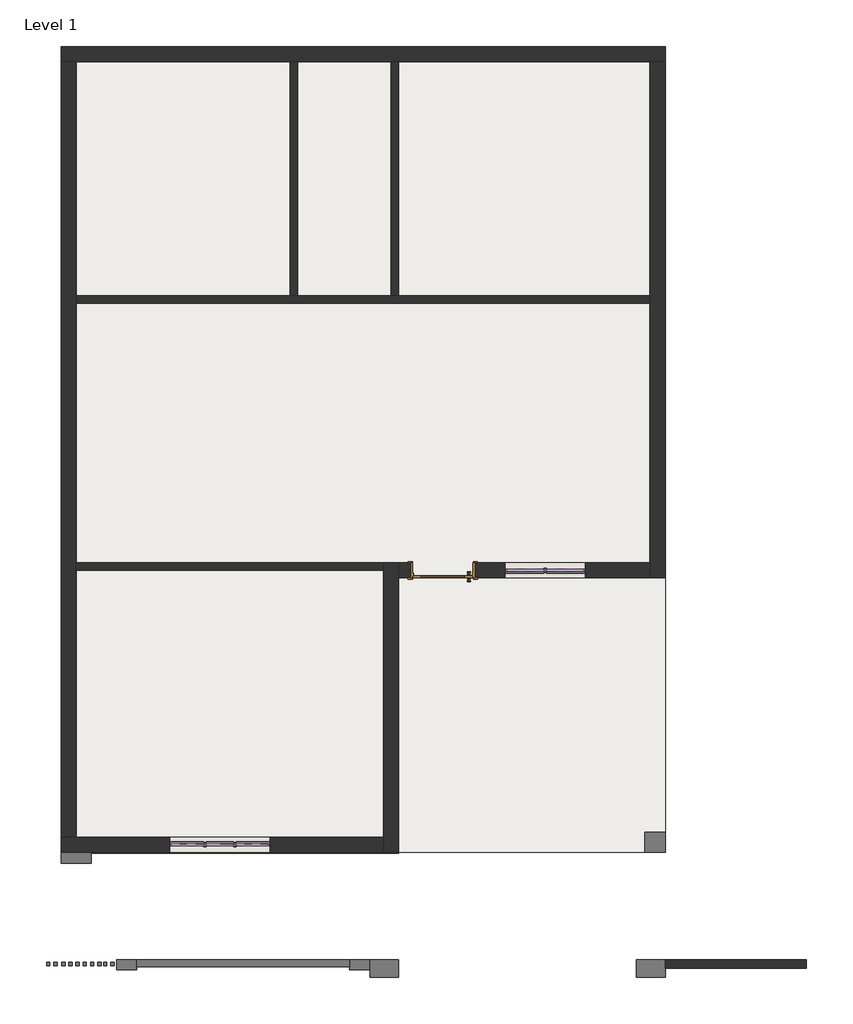
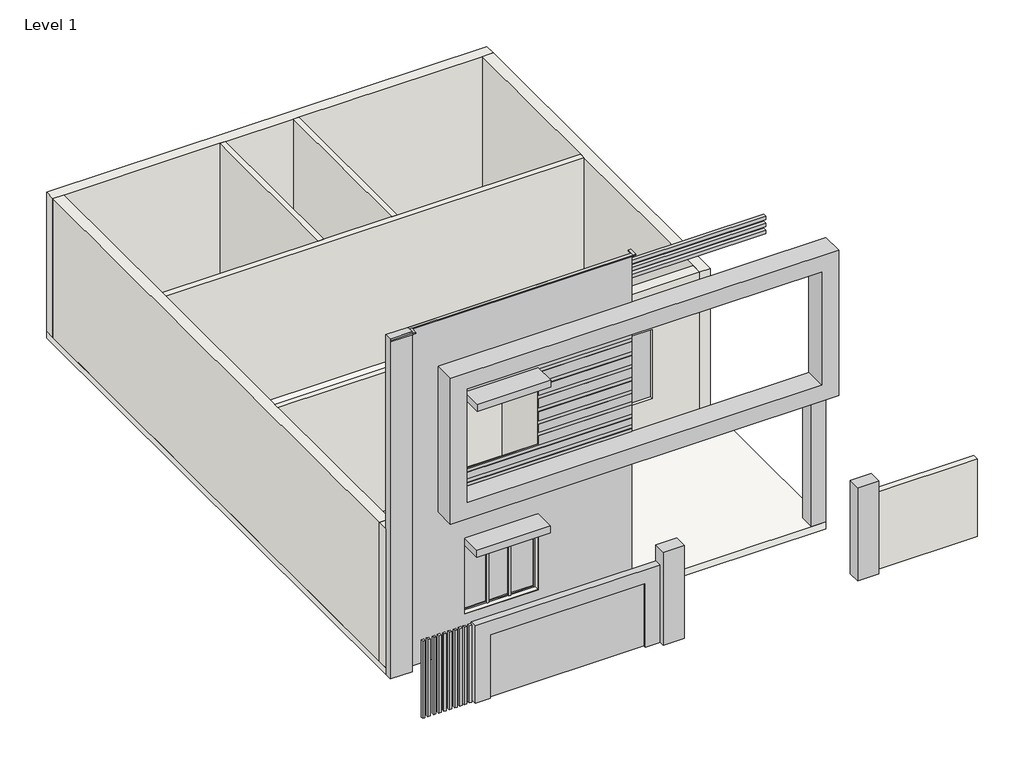
# One storey: 17 members, 11 walls, 5 plates, 4 proxies, 1 door, 1 slab.
"""IFC4 building model written with IfcOpenShell, lengths in millimetres."""

from ifc_helpers import new_model, si_unit, frame, origin, origin_with_axes, place, context, project, spatial, polyline, outline, extrude, faceted_brep, transform, mapped, element, save
from components import generic_models_62b69d9f, generic_models_1_generic_models_1_b53c1211, generic_models_2_generic_models_2_c6cf683d, wall_ext_wall_ext_517f0dc9, door_3b97b8e7, member_d76f7ec7, member_8b4722c0, member_5dd0e0a2, member_31f2b2ad, member_155beb68, system_panel_glazed_7a35cff4, system_panel_glazed_49ff1c72, system_panel_glazed_817050b2

model = new_model("IFC4")

# Units and contexts
model_context = context("Model", 3, world=origin())
ifc_project = project(units=[si_unit("LENGTHUNIT", "METRE", prefix="MILLI")], contexts=[model_context])

# Site, building, storey
site = spatial("IfcSite", under=ifc_project)
building = spatial("IfcBuilding", under=site)
storey = spatial("IfcBuildingStorey", under=building, Name="Level 1", Elevation=0.0)

# Proxies
placement = place(None, origin())
generic_models_shape = generic_models_62b69d9f(model_context)
element("IfcBuildingElementProxy", 1, Name="Generic Models", at=placement, inside=storey, context=model_context, shape_type="MappedRepresentation", body=[
    mapped(generic_models_shape, transform((0.0, 0.0, 0.0), x_axis=(1.0, 0.0, 0.0), y_axis=(0.0, 1.0, 0.0), z_axis=(0.0, 0.0, 1.0))),
])
generic_models_1_generic_models_1_shape = generic_models_1_generic_models_1_b53c1211(model_context)
element("IfcBuildingElementProxy", 2, Name="Generic Models 1 : Generic Models 1", ObjectType="Generic Models 1 : Generic Models 1", at=placement, inside=storey, context=model_context, shape_type="MappedRepresentation", body=[
    mapped(generic_models_1_generic_models_1_shape, transform((0.0, 0.0, 0.0), x_axis=(1.0, 0.0, 0.0), y_axis=(0.0, 1.0, 0.0), z_axis=(0.0, 0.0, 1.0))),
])
generic_models_2_generic_models_2_shape = generic_models_2_generic_models_2_c6cf683d(model_context)
element("IfcBuildingElementProxy", 3, Name="Generic Models 2 : Generic Models 2", ObjectType="Generic Models 2 : Generic Models 2", at=placement, inside=storey, context=model_context, shape_type="MappedRepresentation", body=[
    mapped(generic_models_2_generic_models_2_shape, transform((0.0, 0.0, 0.0), x_axis=(1.0, 0.0, 0.0), y_axis=(0.0, 1.0, 0.0), z_axis=(0.0, 0.0, 1.0))),
])
wall_ext_wall_ext_shape = wall_ext_wall_ext_517f0dc9(model_context)
element("IfcBuildingElementProxy", 4, Name="wall ext : wall ext", ObjectType="wall ext : wall ext", at=placement, inside=storey, context=model_context, shape_type="MappedRepresentation", body=[
    mapped(wall_ext_wall_ext_shape, transform((0.0, 0.0, 0.0), x_axis=(1.0, 0.0, 0.0), y_axis=(0.0, 1.0, 0.0), z_axis=(0.0, 0.0, 1.0))),
])

# Door
door_shape = door_3b97b8e7(model_context)
element("IfcDoor", 5, ObjectType="Door-Interior-Single-1_Panel-Wood : 36\" x 84\"", at=placement, inside=storey, context=model_context, shape_type="MappedRepresentation", body=[
    mapped(door_shape, transform((-7775.8551496, 2378.027641, 0.0), x_axis=(-1.0, 0.0, 0.0), y_axis=(0.0, -1.0, 0.0), z_axis=(0.0, 0.0, 1.0))),
])

# Members
member_shape = member_d76f7ec7(model_context)
element("IfcMember", 6, ObjectType="Rectangular Mullion : 1\" Square", at=placement, inside=storey, context=model_context, shape_type="MappedRepresentation", body=[
    mapped(member_shape, transform((-11916.0551496, -1771.697359, 2133.6), x_axis=(-1.0, 0.0, 0.0), y_axis=(0.0, -1.0, 0.0), z_axis=(0.0, 0.0, 1.0))),
])
element("IfcMember", 7, ObjectType="Rectangular Mullion : 1\" Square", at=placement, inside=storey, context=model_context, shape_type="MappedRepresentation", body=[
    mapped(member_shape, transform((-5616.8551496, 2381.202641, 2133.6), x_axis=(1.0, 0.0, 0.0), y_axis=(0.0, 1.0, 0.0), z_axis=(0.0, 0.0, 1.0))),
])
element("IfcMember", 8, ObjectType="Rectangular Mullion : 1\" Square", at=placement, inside=storey, context=model_context, shape_type="MappedRepresentation", body=[
    mapped(member_shape, transform((-10392.0551496, -1771.697359, 609.6), x_axis=(1.0, 0.0, 0.0), y_axis=(0.0, -1.0, 0.0), z_axis=(0.0, 0.0, -1.0))),
])
element("IfcMember", 9, ObjectType="Rectangular Mullion : 1\" Square", at=placement, inside=storey, context=model_context, shape_type="MappedRepresentation", body=[
    mapped(member_shape, transform((-6836.0551496, 2381.202641, 609.6), x_axis=(-1.0, 0.0, 0.0), y_axis=(0.0, 1.0, 0.0), z_axis=(0.0, 0.0, -1.0))),
])
member_2_shape = member_8b4722c0(model_context)
element("IfcMember", 10, ObjectType="Rectangular Mullion : 1\" Square", at=placement, inside=storey, context=model_context, shape_type="MappedRepresentation", body=[
    mapped(member_2_shape, transform((-10417.4551496, -1771.697359, 2133.6), x_axis=(0.0, 0.0, 1.0), y_axis=(0.0, -1.0, 0.0), z_axis=(1.0, 0.0, 0.0))),
])
element("IfcMember", 11, ObjectType="Rectangular Mullion : 1\" Square", at=placement, inside=storey, context=model_context, shape_type="MappedRepresentation", body=[
    mapped(member_2_shape, transform((-11401.7051496, -1771.697359, 2133.6), x_axis=(0.0, 0.0, 1.0), y_axis=(0.0, -1.0, 0.0), z_axis=(1.0, 0.0, 0.0))),
])
element("IfcMember", 12, ObjectType="Rectangular Mullion : 1\" Square", at=placement, inside=storey, context=model_context, shape_type="MappedRepresentation", body=[
    mapped(member_2_shape, transform((-11890.6551496, -1771.697359, 609.6), x_axis=(0.0, 0.0, -1.0), y_axis=(0.0, -1.0, 0.0), z_axis=(-1.0, 0.0, 0.0))),
])
element("IfcMember", 13, ObjectType="Rectangular Mullion : 1\" Square", at=placement, inside=storey, context=model_context, shape_type="MappedRepresentation", body=[
    mapped(member_2_shape, transform((-10906.4051496, -1771.697359, 609.6), x_axis=(0.0, 0.0, -1.0), y_axis=(0.0, -1.0, 0.0), z_axis=(-1.0, 0.0, 0.0))),
])
member_3_shape = member_5dd0e0a2(model_context)
element("IfcMember", 14, ObjectType="Rectangular Mullion : 1\" Square", at=placement, inside=storey, context=model_context, shape_type="MappedRepresentation", body=[
    mapped(member_3_shape, transform((-11363.6051496, -1771.697359, 609.6), x_axis=(0.0, 0.0, -1.0), y_axis=(0.0, -1.0, 0.0), z_axis=(-1.0, 0.0, 0.0))),
])
element("IfcMember", 15, ObjectType="Rectangular Mullion : 1\" Square", at=placement, inside=storey, context=model_context, shape_type="MappedRepresentation", body=[
    mapped(member_3_shape, transform((-10944.5051496, -1771.697359, 2133.6), x_axis=(0.0, 0.0, 1.0), y_axis=(0.0, -1.0, 0.0), z_axis=(1.0, 0.0, 0.0))),
])
member_4_shape = member_31f2b2ad(model_context)
element("IfcMember", 16, ObjectType="Rectangular Mullion : 1\" Square", at=placement, inside=storey, context=model_context, shape_type="MappedRepresentation", body=[
    mapped(member_4_shape, transform((-6810.6551496, 2381.202641, 2133.6), x_axis=(0.0, 0.0, 1.0), y_axis=(0.0, 1.0, 0.0), z_axis=(-1.0, 0.0, 0.0))),
])
element("IfcMember", 17, ObjectType="Rectangular Mullion : 1\" Square", at=placement, inside=storey, context=model_context, shape_type="MappedRepresentation", body=[
    mapped(member_4_shape, transform((-6207.4051496, 2381.202641, 2133.6), x_axis=(0.0, 0.0, 1.0), y_axis=(0.0, 1.0, 0.0), z_axis=(-1.0, 0.0, 0.0))),
])
element("IfcMember", 18, ObjectType="Rectangular Mullion : 1\" Square", at=placement, inside=storey, context=model_context, shape_type="MappedRepresentation", body=[
    mapped(member_4_shape, transform((-5642.2551496, 2381.202641, 609.6), x_axis=(0.0, 0.0, -1.0), y_axis=(0.0, 1.0, 0.0), z_axis=(1.0, 0.0, 0.0))),
])
element("IfcMember", 19, ObjectType="Rectangular Mullion : 1\" Square", at=placement, inside=storey, context=model_context, shape_type="MappedRepresentation", body=[
    mapped(member_4_shape, transform((-6245.5051496, 2381.202641, 609.6), x_axis=(0.0, 0.0, -1.0), y_axis=(0.0, 1.0, 0.0), z_axis=(1.0, 0.0, 0.0))),
])
member_5_shape = member_155beb68(model_context)
element("IfcMember", 20, ObjectType="Rectangular Mullion : 1.5\" x 2.5\" rectangular", at=placement, inside=storey, context=model_context, shape_type="MappedRepresentation", body=[
    mapped(member_5_shape, transform((-11382.6551496, -1771.697359, 609.6), x_axis=(1.0, 0.0, 0.0), y_axis=(0.0, -1.0, 0.0), z_axis=(0.0, 0.0, -1.0))),
])
element("IfcMember", 21, ObjectType="Rectangular Mullion : 1.5\" x 2.5\" rectangular", at=placement, inside=storey, context=model_context, shape_type="MappedRepresentation", body=[
    mapped(member_5_shape, transform((-10925.4551496, -1771.697359, 609.6), x_axis=(1.0, 0.0, 0.0), y_axis=(0.0, -1.0, 0.0), z_axis=(0.0, 0.0, -1.0))),
])
element("IfcMember", 22, ObjectType="Rectangular Mullion : 1.5\" x 2.5\" rectangular", at=placement, inside=storey, context=model_context, shape_type="MappedRepresentation", body=[
    mapped(member_5_shape, transform((-6226.4551496, 2381.202641, 609.6), x_axis=(-1.0, 0.0, 0.0), y_axis=(0.0, 1.0, 0.0), z_axis=(0.0, 0.0, -1.0))),
])

# Plates
system_panel_glazed_shape = system_panel_glazed_7a35cff4(model_context)
element("IfcPlate", 23, ObjectType="System Panel : Glazed", at=placement, inside=storey, context=model_context, shape_type="MappedRepresentation", body=[
    mapped(system_panel_glazed_shape, transform((-11658.8801496, -1771.697359, 609.6), x_axis=(1.0, 0.0, 0.0), y_axis=(0.0, 1.0, 0.0), z_axis=(0.0, 0.0, 1.0))),
])
element("IfcPlate", 24, ObjectType="System Panel : Glazed", at=placement, inside=storey, context=model_context, shape_type="MappedRepresentation", body=[
    mapped(system_panel_glazed_shape, transform((-10649.2301496, -1771.697359, 609.6), x_axis=(1.0, 0.0, 0.0), y_axis=(0.0, 1.0, 0.0), z_axis=(0.0, 0.0, 1.0))),
])
system_panel_glazed_2_shape = system_panel_glazed_49ff1c72(model_context)
element("IfcPlate", 25, ObjectType="System Panel : Glazed", at=placement, inside=storey, context=model_context, shape_type="MappedRepresentation", body=[
    mapped(system_panel_glazed_2_shape, transform((-11154.0551496, -1771.697359, 609.6), x_axis=(1.0, 0.0, 0.0), y_axis=(0.0, 1.0, 0.0), z_axis=(0.0, 0.0, 1.0))),
])
system_panel_glazed_3_shape = system_panel_glazed_817050b2(model_context)
element("IfcPlate", 26, ObjectType="System Panel : Glazed", at=placement, inside=storey, context=model_context, shape_type="MappedRepresentation", body=[
    mapped(system_panel_glazed_3_shape, transform((-5912.1301496, 2381.202641, 609.6), x_axis=(-1.0, 0.0, 0.0), y_axis=(0.0, -1.0, 0.0), z_axis=(0.0, 0.0, 1.0))),
])
element("IfcPlate", 27, ObjectType="System Panel : Glazed", at=placement, inside=storey, context=model_context, shape_type="MappedRepresentation", body=[
    mapped(system_panel_glazed_3_shape, transform((-6540.7801496, 2381.202641, 609.6), x_axis=(-1.0, 0.0, 0.0), y_axis=(0.0, -1.0, 0.0), z_axis=(0.0, 0.0, 1.0))),
])

# Slab
element("IfcSlab", 28, ObjectType="6\" floor", at=placement, inside=storey, context=model_context, shape_type="SweptSolid", body=[
    extrude(outline(polyline([(-4410.3551496, 10306.002641), (-4410.3551496, -1885.997359), (-13554.3551496, -1885.997359), (-13554.3551496, 10306.002641), (-4410.3551496, 10306.002641)])), frame((0.0, 0.0, -152.4), z_axis=(0.0, 0.0, 1.0), x_axis=(1.0, 0.0, 0.0)), (0.0, 0.0, 1.0), 152.4),
])

# Walls
element("IfcWall", 29, ObjectType="4.5\" INNER WALL", at=placement, inside=storey, context=model_context, shape_type="SweptSolid", body=[
    extrude(outline(polyline([(-13325.7551496, 2495.502641), (-8677.5551496, 2495.502641), (-8677.5551496, 2381.202641), (-13325.7551496, 2381.202641), (-13325.7551496, 2495.502641)])), origin_with_axes(), (0.0, 0.0, 1.0), 3048.0),
])
element("IfcWall", 30, ObjectType="4.5\" INNER WALL", at=placement, inside=storey, context=model_context, shape_type="Brep", body=[
    faceted_brep([(-13325.7551496, 6419.802641, 0.0), (-4638.9551496, 6419.802641, 0.0), (-4638.9551496, 6419.802641, 3048.0), (-13325.7551496, 6419.802641, 3048.0), (-13325.7551496, 6534.102641, 0.0), (-13325.7551496, 6534.102641, 3048.0), (-10087.2551496, 6534.102641, 3048.0), (-9972.9551496, 6534.102641, 3048.0), (-8563.2551496, 6534.102641, 3048.0), (-8448.9551496, 6534.102641, 3048.0), (-4638.9551496, 6534.102641, 3048.0), (-4638.9551496, 6534.102641, 0.0), (-8448.9551496, 6534.102641, 0.0), (-8563.2551496, 6534.102641, 0.0), (-9972.9551496, 6534.102641, 0.0), (-10087.2551496, 6534.102641, 0.0)], [[[0, 1, 2, 3]], [[4, 5, 6, 7, 8, 9, 10, 11, 12, 13, 14, 15]], [[1, 0, 4, 15, 14, 13, 12, 11]], [[3, 2, 10, 9, 8, 7, 6, 5]], [[2, 1, 11, 10]], [[0, 3, 5, 4]]]),
])
element("IfcWall", 31, ObjectType="4.5\" INNER WALL", at=placement, inside=storey, context=model_context, shape_type="SweptSolid", body=[
    extrude(outline(polyline([(-9972.9551496, 10077.402641), (-9972.9551496, 6534.102641), (-10087.2551496, 6534.102641), (-10087.2551496, 10077.402641), (-9972.9551496, 10077.402641)])), origin_with_axes(), (0.0, 0.0, 1.0), 3048.0),
])
element("IfcWall", 32, ObjectType="4.5\" INNER WALL", at=placement, inside=storey, context=model_context, shape_type="SweptSolid", body=[
    extrude(outline(polyline([(-8448.9551496, 10077.402641), (-8448.9551496, 6534.102641), (-8563.2551496, 6534.102641), (-8563.2551496, 10077.402641), (-8448.9551496, 10077.402641)])), origin_with_axes(), (0.0, 0.0, 1.0), 3048.0),
])
element("IfcWall", 33, ObjectType="9\" WALL", at=placement, inside=storey, context=model_context, shape_type="Brep", body=[
    faceted_brep([(-13554.3551496, 10077.402641, 0.0), (-13325.7551496, 10077.402641, 0.0), (-10087.2551496, 10077.402641, 0.0), (-9972.9551496, 10077.402641, 0.0), (-8563.2551496, 10077.402641, 0.0), (-8448.9551496, 10077.402641, 0.0), (-4638.9551496, 10077.402641, 0.0), (-4410.3551496, 10077.402641, 0.0), (-4410.3551496, 10077.402641, 3048.0), (-4638.9551496, 10077.402641, 3048.0), (-8448.9551496, 10077.402641, 3048.0), (-8563.2551496, 10077.402641, 3048.0), (-9972.9551496, 10077.402641, 3048.0), (-10087.2551496, 10077.402641, 3048.0), (-13325.7551496, 10077.402641, 3048.0), (-13554.3551496, 10077.402641, 3048.0), (-13554.3551496, 10306.002641, 0.0), (-13554.3551496, 10306.002641, 3048.0), (-4410.3551496, 10306.002641, 3048.0), (-4410.3551496, 10306.002641, 0.0)], [[[0, 1, 2, 3, 4, 5, 6, 7, 8, 9, 10, 11, 12, 13, 14, 15]], [[16, 17, 18, 19]], [[7, 6, 5, 4, 3, 2, 1, 0, 16, 19]], [[15, 14, 13, 12, 11, 10, 9, 8, 18, 17]], [[8, 7, 19, 18]], [[0, 15, 17, 16]]]),
])
element("IfcWall", 34, ObjectType="9\" WALL", at=placement, inside=storey, context=model_context, shape_type="Brep", body=[
    faceted_brep([(-4638.9551496, 10077.402641, 0.0), (-4638.9551496, 6534.102641, 0.0), (-4638.9551496, 6419.802641, 0.0), (-4638.9551496, 2495.502641, 0.0), (-4638.9551496, 2266.902641, 0.0), (-4638.9551496, 2266.902641, 3048.0), (-4638.9551496, 2495.502641, 3048.0), (-4638.9551496, 6419.802641, 3048.0), (-4638.9551496, 6534.102641, 3048.0), (-4638.9551496, 10077.402641, 3048.0), (-4410.3551496, 10077.402641, 0.0), (-4410.3551496, 10077.402641, 3048.0), (-4410.3551496, 2266.902641, 3048.0), (-4410.3551496, 2266.902641, 0.0)], [[[0, 1, 2, 3, 4, 5, 6, 7, 8, 9]], [[10, 11, 12, 13]], [[4, 3, 2, 1, 0, 10, 13]], [[9, 8, 7, 6, 5, 12, 11]], [[0, 9, 11, 10]], [[5, 4, 13, 12]]]),
])
element("IfcWall", 35, ObjectType="9\" WALL", at=placement, inside=storey, context=model_context, shape_type="Brep", body=[
    faceted_brep([(-13325.7551496, -1657.397359, 0.0), (-13325.7551496, 2381.202641, 0.0), (-13325.7551496, 2495.502641, 0.0), (-13325.7551496, 6419.802641, 0.0), (-13325.7551496, 6534.102641, 0.0), (-13325.7551496, 10077.402641, 0.0), (-13325.7551496, 10077.402641, 3048.0), (-13325.7551496, 6534.102641, 3048.0), (-13325.7551496, 6419.802641, 3048.0), (-13325.7551496, 2495.502641, 3048.0), (-13325.7551496, 2381.202641, 3048.0), (-13325.7551496, -1657.397359, 3048.0), (-13554.3551496, -1657.397359, 0.0), (-13554.3551496, -1657.397359, 3048.0), (-13554.3551496, 10077.402641, 3048.0), (-13554.3551496, 10077.402641, 0.0)], [[[0, 1, 2, 3, 4, 5, 6, 7, 8, 9, 10, 11]], [[12, 13, 14, 15]], [[5, 4, 3, 2, 1, 0, 12, 15]], [[11, 10, 9, 8, 7, 6, 14, 13]], [[0, 11, 13, 12]], [[6, 5, 15, 14]]]),
])
element("IfcWall", 36, ObjectType="9\" WALL", at=placement, inside=storey, context=model_context, shape_type="Brep", body=[
    faceted_brep([(-8448.9551496, -1885.997359, 0.0), (-8448.9551496, 2266.902641, 0.0), (-8448.9551496, 2495.502641, 0.0), (-8448.9551496, 2495.502641, 3048.0), (-8448.9551496, 2266.902641, 3048.0), (-8448.9551496, -1885.997359, 3048.0), (-8677.5551496, -1885.997359, 0.0), (-8677.5551496, -1885.997359, 3048.0), (-8677.5551496, -1657.397359, 3048.0), (-8677.5551496, 2381.202641, 3048.0), (-8677.5551496, 2495.502641, 3048.0), (-8677.5551496, 2495.502641, 0.0), (-8677.5551496, 2381.202641, 0.0), (-8677.5551496, -1657.397359, 0.0)], [[[0, 1, 2, 3, 4, 5]], [[6, 7, 8, 9, 10, 11, 12, 13]], [[2, 1, 0, 6, 13, 12, 11]], [[5, 4, 3, 10, 9, 8, 7]], [[3, 2, 11, 10]], [[0, 5, 7, 6]]]),
])
element("IfcWall", 37, ObjectType="9\" WALL", at=placement, inside=storey, context=model_context, shape_type="SweptSolid", body=[
    extrude(outline(polyline([(3048.0, -4638.9551496), (3048.0, -8448.9551496), (0.0, -8448.9551496), (0.0, -8258.4551496), (2159.0, -8258.4551496), (2159.0, -7293.2551496), (0.0, -7293.2551496), (0.0, -4638.9551496), (3048.0, -4638.9551496)]), holes=[polyline([(2133.6, -5616.8551496), (609.6, -5616.8551496), (609.6, -6836.0551496), (2133.6, -6836.0551496), (2133.6, -5616.8551496)])]), frame((0.0, 2266.902641, 0.0), z_axis=(0.0, 1.0, 0.0), x_axis=(0.0, 0.0, 1.0)), (0.0, 0.0, 1.0), 228.6),
])
element("IfcWall", 38, ObjectType="9\" WALL", at=placement, inside=storey, context=model_context, shape_type="Brep", body=[
    faceted_brep([(-8677.5551496, -1657.397359, 0.0), (-13325.7551496, -1657.397359, 0.0), (-13554.3551496, -1657.397359, 0.0), (-13554.3551496, -1657.397359, 3048.0), (-13325.7551496, -1657.397359, 3048.0), (-8677.5551496, -1657.397359, 3048.0), (-11916.0551496, -1657.397359, 2133.6), (-11916.0551496, -1657.397359, 609.6), (-10392.0551496, -1657.397359, 609.6), (-10392.0551496, -1657.397359, 2133.6), (-13554.3551496, -1885.997359, 0.0), (-8677.5551496, -1885.997359, 0.0), (-8677.5551496, -1885.997359, 3048.0), (-13554.3551496, -1885.997359, 3048.0), (-11916.0551496, -1885.997359, 609.6), (-11916.0551496, -1885.997359, 2133.6), (-10392.0551496, -1885.997359, 2133.6), (-10392.0551496, -1885.997359, 609.6)], [[[0, 1, 2, 3, 4, 5], [6, 7, 8, 9]], [[10, 11, 12, 13], [14, 15, 16, 17]], [[2, 1, 0, 11, 10]], [[5, 4, 3, 13, 12]], [[3, 2, 10, 13]], [[0, 5, 12, 11]], [[14, 7, 6, 15]], [[15, 6, 9, 16]], [[16, 9, 8, 17]], [[7, 14, 17, 8]]]),
])
element("IfcWall", 39, ObjectType="Generic - 5\"", at=placement, inside=storey, context=model_context, shape_type="SweptSolid", body=[
    extrude(outline(polyline([(-2276.7551496, -3638.597359), (-4410.3551496, -3638.597359), (-4410.3551496, -3511.597359), (-2276.7551496, -3511.597359), (-2276.7551496, -3638.597359)])), origin_with_axes(), (0.0, 0.0, 1.0), 1698.9467307),
])

save(model, "model.ifc")

# Revit data of these elements
# Type "Door-Interior-Single-1_Panel-Wood : 36\" x 84\""
#   Type Mark = "8"
#   Assembly Code = "C1020300"
#   Analytic Construction = "Wooden"
#   Top Rail = 0' - 4 11/16"
#   Thickness = 0' - 1 3/8"
#   Thermal Resistance (R) = 2.5876 (h·ft²·°F)/BTU
#   Swing Angle [instance default] = 90.00°
#   Stiles = 0' - 4 3/4"
#   Rough Width = 3' - 2"
#   Rough Height = 7' - 1"
#   Height = 7' - 0"
#   Width = 3' - 0"
#   Heat Transfer Coefficient (U) = 0.3865 BTU/(h·ft²·°F)
#   Bottom Rail = 0' - 9 1/8"
#   Trim Material = Cherry
#   Panel Material = door
#   Frame Material = door
#   Door Handle Material = Aluminum
#   Visual Light Transmittance = 0
#   Solar Heat Gain Coefficient = 0
#   Wall Closure = (empty or 0)
#   Function = (empty or 0)
# Type "Rectangular Mullion : 1\" Square"
#   built-in parameter 1007304 = 0.0833333 (stored number, unit not read)
#   built-in parameter 1007301 = 0.0416667 (stored number, unit not read)
#   built-in parameter 1007300 = 0.0416667 (stored number, unit not read)
# Type "Rectangular Mullion : 1.5\" x 2.5\" rectangular"
#   built-in parameter 1007304 = 0.208333 (stored number, unit not read)
#   built-in parameter 1007301 = 0.0625 (stored number, unit not read)
#   built-in parameter 1007300 = 0.0625 (stored number, unit not read)
# Type "System Panel : Glazed"
#   Construction Type Id = "GSP4R"
#   Analytic Construction = "1/8 in Pilkington single glazing"
#   Visual Light Transmittance = 0.9
#   Solar Heat Gain Coefficient = 0.86
#   Heat Transfer Coefficient (U) = 1.18115 BTU/(h·ft²·°F)
#   Define Thermal Properties by = 1
# Type "6\" floor"
#   Assembly Code = "B1010"
#   Function = 0
#   Layers, outside or top first: 0' - 6" no material (function 1)
# Type "4.5\" INNER WALL"
#   Assembly Code = "B2010"
#   Layers, outside or top first: 0' - 4 1/2" "Damp-proofing" (function 1)
# Type "9\" WALL"
#   Assembly Code = "B2010"
#   Layers, outside or top first: 0' - 9" "Analytical Surface - Exterior Walls" (function 1)
# Type "Generic - 5\""
#   Assembly Code = "B2010"
#   Layers, outside or top first: 0' - 5" "Gypsum Wall Board" (function 1)
# Element 1 (IfcBuildingElementProxy)
#   Phase Created = New Construction
#   Materials on its faces: "Roofing, EPDM Membrane", "wall", "Gypsum Wall Board", "Door - Frame"
# Element 2 (IfcBuildingElementProxy, "Generic Models 1 : Generic Models 1")
#   Phase Created = New Construction
#   Materials on its faces: "Gypsum Wall Board"
# Element 3 (IfcBuildingElementProxy, "Generic Models 2 : Generic Models 2")
#   Phase Created = New Construction
# Element 4 (IfcBuildingElementProxy, "wall ext : wall ext")
#   Phase Created = New Construction
#   Materials on its faces: "Door - Frame", "Damp-proofing", "wall"
# Element 5 (IfcDoor, "Door-Interior-Single-1_Panel-Wood : 36\" x 84\"")
#   Swing Angle = 90.00°
#   Phase Created = New Construction
#   Materials on its faces: "Aluminum", "door", "Cherry"
# Elements 6, 7, 8, 9, 10, 11, 12, 13, 14, 15, 16, 17, 18, 19 (IfcMember, "Rectangular Mullion : 1\" Square")
#   Phase Created = New Construction
# Elements 20, 21, 22 (IfcMember, "Rectangular Mullion : 1.5\" x 2.5\" rectangular")
#   Phase Created = New Construction
#   Materials on its faces: "mullions"
# Elements 23, 24, 25, 26, 27 (IfcPlate, "System Panel : Glazed")
#   Phase Created = New Construction
#   Materials on its faces: "Glass"
# Element 28 (IfcSlab, "6\" floor")
#   Height Offset From Level = 0' - 0"
#   Phase Created = New Construction
#   Materials on its faces: "Default Floor"
# Elements 29, 30, 31, 32 (IfcWall, "4.5\" INNER WALL")
#   Top Offset = 0' - 0"
#   Base Offset = 0' - 0"
#   wall height = 10' - 0"
#   Phase Created = New Construction
#   Base Constraint = Level 1
#   Top Constraint = Level 2
#   Materials on its faces: "Damp-proofing"
# Elements 33, 34, 35, 36, 37, 38 (IfcWall, "9\" WALL")
#   Top Offset = 0' - 0"
#   Base Offset = 0' - 0"
#   wall height = 10' - 0"
#   Phase Created = New Construction
#   Base Constraint = Level 1
#   Top Constraint = Level 2
#   Materials on its faces: "Analytical Surface - Exterior Walls"
# Element 39 (IfcWall, "Generic - 5\"")
#   Top Offset = -4' - 5.11233"
#   Base Offset = 0' - 0"
#   wall height = 5' - 6.88767"
#   Phase Created = New Construction
#   Base Constraint = Level 1
#   Top Constraint = Level 2
#   Materials on its faces: "Gypsum Wall Board"
# Materials
#   "Cherry": class "Wood", colour RGB 226 177 128, transparency 0, Description = "Prunus Serotina", Cost = 0
#   "door": class "Generic", colour RGB 120 120 120, transparency 0, Cost = 0
#   "Aluminum": class "Metal", colour RGB 247 247 247, transparency 0, Description = "Aluminum 6061", Cost = 0
#   "Damp-proofing": class "Generic", colour RGB 127 127 127, transparency 0, Description = "Damp-proofing", Cost = 0
#   "Analytical Surface - Exterior Walls": colour RGB 133 178 44, transparency 0.5, Cost = 0
#   "Gypsum Wall Board": class "Generic", colour RGB 127 127 127, transparency 0, Description = "Gypsum Wall Board", Cost = 0
#   "Roofing, EPDM Membrane": class "Generic", colour RGB 127 127 127, transparency 0, Description = "EPDM roof membrane", Cost = 0
#   "wall": class "Generic", colour RGB 120 120 120, transparency 0, Cost = 0
#   "Door - Frame": colour RGB 118 70 51, transparency 0, Cost = 0
#   "mullions": class "Generic", colour RGB 120 120 120, transparency 0, Cost = 0
#   "Glass": class "Glass", colour RGB 0 128 192, transparency 0.75, Description = "Soda Lime Glass", Cost = 0
#   "Default Floor": colour RGB 128 128 128, transparency 0, Cost = 0
